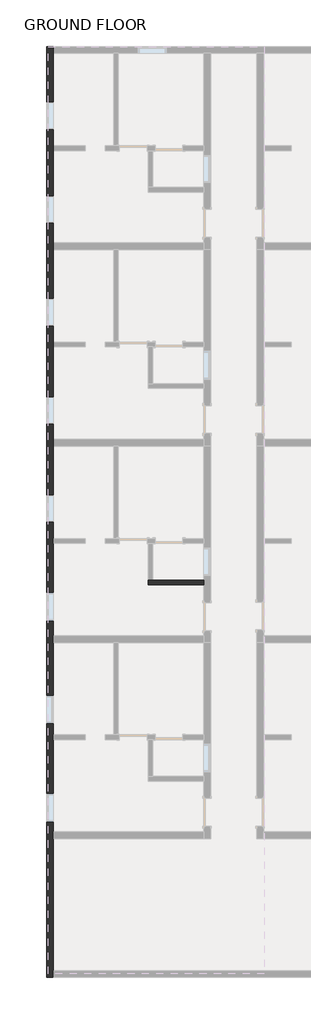
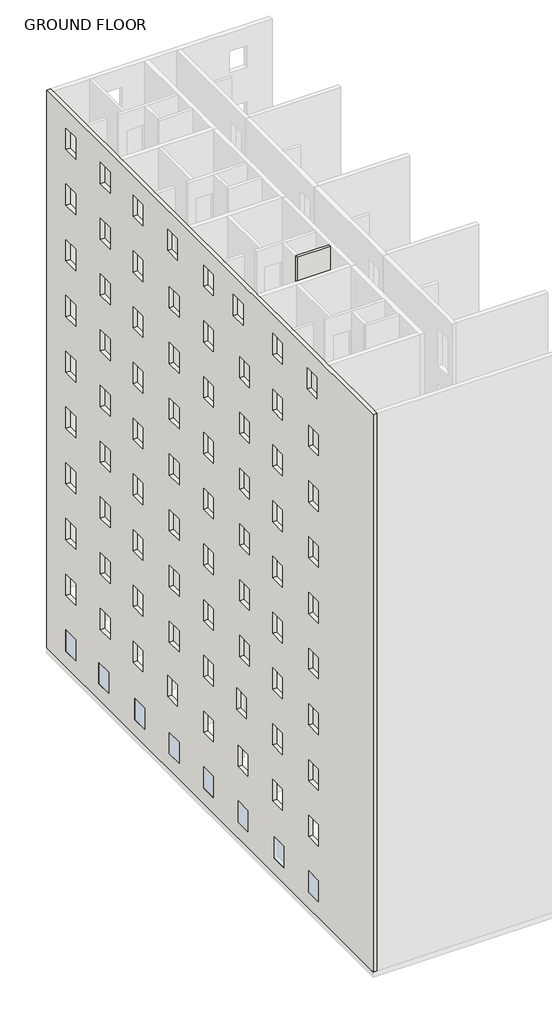
# One storey, part 2 of 7: 2 walls.
"""IFC4 building model written with IfcOpenShell, lengths in millimetres."""

from ifc_helpers import new_model, si_unit, origin, place, context, project, spatial, faceted_brep, element, save

model = new_model("IFC4")

# Units and contexts
model_context = context("Model", 3, world=origin())
ifc_project = project(units=[si_unit("LENGTHUNIT", "METRE", prefix="MILLI")], contexts=[model_context])

# Site, building, storey
site = spatial("IfcSite", under=ifc_project)
building = spatial("IfcBuilding", under=site)
storey = spatial("IfcBuildingStorey", under=building, Name="GROUND FLOOR", Elevation=0.0)

# Walls
placement = place(None, origin())
element("IfcWall", 1, ObjectType="INNER WALL 2", at=placement, inside=storey, context=model_context, shape_type="Brep", body=[
    faceted_brep([(-7539.4902461, -2297.1289408, 0.0), (-9215.8902461, -2297.1289408, 0.0), (-9368.2902461, -2297.1289408, 0.0), (-9368.2902461, -2297.1289408, 32004.0), (-9215.8902461, -2297.1289408, 32004.0), (-7539.4902461, -2297.1289408, 32004.0), (-7539.4902461, -2449.5289408, 0.0), (-7539.4902461, -2449.5289408, 32004.0), (-9368.2902461, -2449.5289408, 32004.0), (-9368.2902461, -2449.5289408, 0.0)], [[[0, 1, 2, 3, 4, 5]], [[6, 7, 8, 9]], [[2, 1, 0, 6, 9]], [[5, 4, 3, 8, 7]], [[0, 5, 7, 6]], [[3, 2, 9, 8]]]),
])
element("IfcWall", 2, ObjectType="OUTER WALL", at=placement, inside=storey, context=model_context, shape_type="Brep", body=[
    faceted_brep([(-12492.4902461, -15403.5289408, 0.0), (-12492.4902461, -15174.9289408, 0.0), (-12492.4902461, -10831.5289408, 0.0), (-12492.4902461, -10602.9289408, 0.0), (-12492.4902461, -7554.9289408, 0.0), (-12492.4902461, -7402.5289408, 0.0), (-12492.4902461, -4354.5289408, 0.0), (-12492.4902461, -4125.9289408, 0.0), (-12492.4902461, -1077.9289408, 0.0), (-12492.4902461, -925.5289408, 0.0), (-12492.4902461, 2122.4710592, 0.0), (-12492.4902461, 2351.0710592, 0.0), (-12492.4902461, 5399.0710592, 0.0), (-12492.4902461, 5551.4710592, 0.0), (-12492.4902461, 8599.4710592, 0.0), (-12492.4902461, 8828.0710592, 0.0), (-12492.4902461, 11876.0710592, 0.0), (-12492.4902461, 12028.4710592, 0.0), (-12492.4902461, 15076.4710592, 0.0), (-12492.4902461, 15305.0710592, 0.0), (-12492.4902461, 15305.0710592, 32004.0), (-12492.4902461, 15076.4710592, 32004.0), (-12492.4902461, 12028.4710592, 32004.0), (-12492.4902461, 11876.0710592, 32004.0), (-12492.4902461, 8828.0710592, 32004.0), (-12492.4902461, 8599.4710592, 32004.0), (-12492.4902461, 5551.4710592, 32004.0), (-12492.4902461, 5399.0710592, 32004.0), (-12492.4902461, 2351.0710592, 32004.0), (-12492.4902461, 2122.4710592, 32004.0), (-12492.4902461, -925.5289408, 32004.0), (-12492.4902461, -1077.9289408, 32004.0), (-12492.4902461, -4125.9289408, 32004.0), (-12492.4902461, -4354.5289408, 32004.0), (-12492.4902461, -7402.5289408, 32004.0), (-12492.4902461, -7554.9289408, 32004.0), (-12492.4902461, -10602.9289408, 32004.0), (-12492.4902461, -10831.5289408, 32004.0), (-12492.4902461, -15174.9289408, 32004.0), (-12492.4902461, -15403.5289408, 32004.0), (-12492.4902461, 13476.2710592, 2133.6), (-12492.4902461, 13476.2710592, 914.4), (-12492.4902461, 12561.8710592, 914.4), (-12492.4902461, 12561.8710592, 2133.6), (-12492.4902461, 10390.1710592, 2133.6), (-12492.4902461, 10390.1710592, 914.4), (-12492.4902461, 9475.7710592, 914.4), (-12492.4902461, 9475.7710592, 2133.6), (-12492.4902461, 6999.2710592, 2133.6), (-12492.4902461, 6999.2710592, 914.4), (-12492.4902461, 6084.8710592, 914.4), (-12492.4902461, 6084.8710592, 2133.6), (-12492.4902461, 3760.7710592, 2133.6), (-12492.4902461, 3760.7710592, 914.4), (-12492.4902461, 2846.3710592, 914.4), (-12492.4902461, 2846.3710592, 2133.6), (-12492.4902461, 522.2710592, 2133.6), (-12492.4902461, 522.2710592, 914.4), (-12492.4902461, -392.1289408, 914.4), (-12492.4902461, -392.1289408, 2133.6), (-12492.4902461, -2716.2289408, 2133.6), (-12492.4902461, -2716.2289408, 914.4), (-12492.4902461, -3630.6289408, 914.4), (-12492.4902461, -3630.6289408, 2133.6), (-12492.4902461, -7021.5289408, 2133.6), (-12492.4902461, -6107.1289408, 2133.6), (-12492.4902461, -6107.1289408, 914.4), (-12492.4902461, -7021.5289408, 914.4), (-12492.4902461, -9345.6289408, 2133.6), (-12492.4902461, -9345.6289408, 914.4), (-12492.4902461, -10260.0289408, 914.4), (-12492.4902461, -10260.0289408, 2133.6), (-12492.4902461, 13476.2710592, 5334.0), (-12492.4902461, 13476.2710592, 4114.8), (-12492.4902461, 12561.8710592, 4114.8), (-12492.4902461, 12561.8710592, 5334.0), (-12492.4902461, 10237.7710592, 5334.0), (-12492.4902461, 10237.7710592, 4114.8), (-12492.4902461, 9323.3710592, 4114.8), (-12492.4902461, 9323.3710592, 5334.0), (-12492.4902461, 7151.6710592, 5334.0), (-12492.4902461, 7151.6710592, 4114.8), (-12492.4902461, 6237.2710592, 4114.8), (-12492.4902461, 6237.2710592, 5334.0), (-12492.4902461, 3913.1710592, 5334.0), (-12492.4902461, 3913.1710592, 4114.8), (-12492.4902461, 2998.7710592, 4114.8), (-12492.4902461, 2998.7710592, 5334.0), (-12492.4902461, 522.2710592, 5334.0), (-12492.4902461, 522.2710592, 4114.8), (-12492.4902461, -392.1289408, 4114.8), (-12492.4902461, -392.1289408, 5334.0), (-12492.4902461, -2716.2289408, 5334.0), (-12492.4902461, -2716.2289408, 4114.8), (-12492.4902461, -3630.6289408, 4114.8), (-12492.4902461, -3630.6289408, 5334.0), (-12492.4902461, -5954.7289408, 5334.0), (-12492.4902461, -5954.7289408, 4114.8), (-12492.4902461, -6869.1289408, 4114.8), (-12492.4902461, -6869.1289408, 5334.0), (-12492.4902461, -9345.6289408, 5334.0), (-12492.4902461, -9345.6289408, 4114.8), (-12492.4902461, -10260.0289408, 4114.8), (-12492.4902461, -10260.0289408, 5334.0), (-12492.4902461, 13476.2710592, 8534.4), (-12492.4902461, 13476.2710592, 7315.2), (-12492.4902461, 12561.8710592, 7315.2), (-12492.4902461, 12561.8710592, 8534.4), (-12492.4902461, 10237.7710592, 8534.4), (-12492.4902461, 10237.7710592, 7315.2), (-12492.4902461, 9323.3710592, 7315.2), (-12492.4902461, 9323.3710592, 8534.4), (-12492.4902461, 7151.6710592, 8534.4), (-12492.4902461, 7151.6710592, 7315.2), (-12492.4902461, 6237.2710592, 7315.2), (-12492.4902461, 6237.2710592, 8534.4), (-12492.4902461, 3760.7710592, 8534.4), (-12492.4902461, 3760.7710592, 7315.2), (-12492.4902461, 2846.3710592, 7315.2), (-12492.4902461, 2846.3710592, 8534.4), (-12492.4902461, 522.2710592, 8534.4), (-12492.4902461, 522.2710592, 7315.2), (-12492.4902461, -392.1289408, 7315.2), (-12492.4902461, -392.1289408, 8534.4), (-12492.4902461, -2563.8289408, 8534.4), (-12492.4902461, -2563.8289408, 7315.2), (-12492.4902461, -3478.2289408, 7315.2), (-12492.4902461, -3478.2289408, 8534.4), (-12492.4902461, -5954.7289408, 8534.4), (-12492.4902461, -5954.7289408, 7315.2), (-12492.4902461, -6869.1289408, 7315.2), (-12492.4902461, -6869.1289408, 8534.4), (-12492.4902461, -9345.6289408, 8534.4), (-12492.4902461, -9345.6289408, 7315.2), (-12492.4902461, -10260.0289408, 7315.2), (-12492.4902461, -10260.0289408, 8534.4), (-12492.4902461, 13476.2710592, 11734.8), (-12492.4902461, 13476.2710592, 10515.6), (-12492.4902461, 12561.8710592, 10515.6), (-12492.4902461, 12561.8710592, 11734.8), (-12492.4902461, 10237.7710592, 11734.8), (-12492.4902461, 10237.7710592, 10515.6), (-12492.4902461, 9323.3710592, 10515.6), (-12492.4902461, 9323.3710592, 11734.8), (-12492.4902461, 7151.6710592, 11734.8), (-12492.4902461, 7151.6710592, 10515.6), (-12492.4902461, 6237.2710592, 10515.6), (-12492.4902461, 6237.2710592, 11734.8), (-12492.4902461, 3760.7710592, 11734.8), (-12492.4902461, 3760.7710592, 10515.6), (-12492.4902461, 2846.3710592, 10515.6), (-12492.4902461, 2846.3710592, 11734.8), (-12492.4902461, 522.2710592, 11734.8), (-12492.4902461, 522.2710592, 10515.6), (-12492.4902461, -392.1289408, 10515.6), (-12492.4902461, -392.1289408, 11734.8), (-12492.4902461, -2868.6289408, 11734.8), (-12492.4902461, -2868.6289408, 10515.6), (-12492.4902461, -3783.0289408, 10515.6), (-12492.4902461, -3783.0289408, 11734.8), (-12492.4902461, -5954.7289408, 11734.8), (-12492.4902461, -5954.7289408, 10515.6), (-12492.4902461, -6869.1289408, 10515.6), (-12492.4902461, -6869.1289408, 11734.8), (-12492.4902461, -9345.6289408, 11734.8), (-12492.4902461, -9345.6289408, 10515.6), (-12492.4902461, -10260.0289408, 10515.6), (-12492.4902461, -10260.0289408, 11734.8), (-12492.4902461, -9345.6289408, 14935.2), (-12492.4902461, -9345.6289408, 13716.0), (-12492.4902461, -10260.0289408, 13716.0), (-12492.4902461, -10260.0289408, 14935.2), (-12492.4902461, -5954.7289408, 14935.2), (-12492.4902461, -5954.7289408, 13716.0), (-12492.4902461, -6869.1289408, 13716.0), (-12492.4902461, -6869.1289408, 14935.2), (-12492.4902461, -2868.6289408, 14935.2), (-12492.4902461, -2868.6289408, 13716.0), (-12492.4902461, -3783.0289408, 13716.0), (-12492.4902461, -3783.0289408, 14935.2), (-12492.4902461, 522.2710592, 14935.2), (-12492.4902461, 522.2710592, 13716.0), (-12492.4902461, -392.1289408, 13716.0), (-12492.4902461, -392.1289408, 14935.2), (-12492.4902461, 3760.7710592, 14935.2), (-12492.4902461, 3760.7710592, 13716.0), (-12492.4902461, 2846.3710592, 13716.0), (-12492.4902461, 2846.3710592, 14935.2), (-12492.4902461, 7151.6710592, 14935.2), (-12492.4902461, 7151.6710592, 13716.0), (-12492.4902461, 6237.2710592, 13716.0), (-12492.4902461, 6237.2710592, 14935.2), (-12492.4902461, 10237.7710592, 14935.2), (-12492.4902461, 10237.7710592, 13716.0), (-12492.4902461, 9323.3710592, 13716.0), (-12492.4902461, 9323.3710592, 14935.2), (-12492.4902461, 13476.2710592, 14935.2), (-12492.4902461, 13476.2710592, 13716.0), (-12492.4902461, 12561.8710592, 13716.0), (-12492.4902461, 12561.8710592, 14935.2), (-12492.4902461, 13476.2710592, 18135.6), (-12492.4902461, 13476.2710592, 16916.4), (-12492.4902461, 12561.8710592, 16916.4), (-12492.4902461, 12561.8710592, 18135.6), (-12492.4902461, 10237.7710592, 18135.6), (-12492.4902461, 10237.7710592, 16916.4), (-12492.4902461, 9323.3710592, 16916.4), (-12492.4902461, 9323.3710592, 18135.6), (-12492.4902461, 7151.6710592, 18135.6), (-12492.4902461, 7151.6710592, 16916.4), (-12492.4902461, 6237.2710592, 16916.4), (-12492.4902461, 6237.2710592, 18135.6), (-12492.4902461, 3760.7710592, 18135.6), (-12492.4902461, 3760.7710592, 16916.4), (-12492.4902461, 2846.3710592, 16916.4), (-12492.4902461, 2846.3710592, 18135.6), (-12492.4902461, 522.2710592, 18135.6), (-12492.4902461, 522.2710592, 16916.4), (-12492.4902461, -392.1289408, 16916.4), (-12492.4902461, -392.1289408, 18135.6), (-12492.4902461, -2868.6289408, 18135.6), (-12492.4902461, -2868.6289408, 16916.4), (-12492.4902461, -3783.0289408, 16916.4), (-12492.4902461, -3783.0289408, 18135.6), (-12492.4902461, -5954.7289408, 18135.6), (-12492.4902461, -5954.7289408, 16916.4), (-12492.4902461, -6869.1289408, 16916.4), (-12492.4902461, -6869.1289408, 18135.6), (-12492.4902461, -9345.6289408, 18135.6), (-12492.4902461, -9345.6289408, 16916.4), (-12492.4902461, -10260.0289408, 16916.4), (-12492.4902461, -10260.0289408, 18135.6), (-12492.4902461, -9345.6289408, 21336.0), (-12492.4902461, -9345.6289408, 20116.8), (-12492.4902461, -10260.0289408, 20116.8), (-12492.4902461, -10260.0289408, 21336.0), (-12492.4902461, -5954.7289408, 21336.0), (-12492.4902461, -5954.7289408, 20116.8), (-12492.4902461, -6869.1289408, 20116.8), (-12492.4902461, -6869.1289408, 21336.0), (-12492.4902461, -2868.6289408, 21336.0), (-12492.4902461, -2868.6289408, 20116.8), (-12492.4902461, -3783.0289408, 20116.8), (-12492.4902461, -3783.0289408, 21336.0), (-12492.4902461, 522.2710592, 21336.0), (-12492.4902461, 522.2710592, 20116.8), (-12492.4902461, -392.1289408, 20116.8), (-12492.4902461, -392.1289408, 21336.0), (-12492.4902461, 3760.7710592, 21336.0), (-12492.4902461, 3760.7710592, 20116.8), (-12492.4902461, 2846.3710592, 20116.8), (-12492.4902461, 2846.3710592, 21336.0), (-12492.4902461, 7151.6710592, 21336.0), (-12492.4902461, 7151.6710592, 20116.8), (-12492.4902461, 6237.2710592, 20116.8), (-12492.4902461, 6237.2710592, 21336.0), (-12492.4902461, 10237.7710592, 21336.0), (-12492.4902461, 10237.7710592, 20116.8), (-12492.4902461, 9323.3710592, 20116.8), (-12492.4902461, 9323.3710592, 21336.0), (-12492.4902461, 13476.2710592, 21336.0), (-12492.4902461, 13476.2710592, 20116.8), (-12492.4902461, 12561.8710592, 20116.8), (-12492.4902461, 12561.8710592, 21336.0), (-12492.4902461, -9345.6289408, 24536.4), (-12492.4902461, -9345.6289408, 23317.2), (-12492.4902461, -10260.0289408, 23317.2), (-12492.4902461, -10260.0289408, 24536.4), (-12492.4902461, -5954.7289408, 24536.4), (-12492.4902461, -5954.7289408, 23317.2), (-12492.4902461, -6869.1289408, 23317.2), (-12492.4902461, -6869.1289408, 24536.4), (-12492.4902461, -2868.6289408, 24536.4), (-12492.4902461, -2868.6289408, 23317.2), (-12492.4902461, -3783.0289408, 23317.2), (-12492.4902461, -3783.0289408, 24536.4), (-12492.4902461, 522.2710592, 24536.4), (-12492.4902461, 522.2710592, 23317.2), (-12492.4902461, -392.1289408, 23317.2), (-12492.4902461, -392.1289408, 24536.4), (-12492.4902461, 3760.7710592, 24536.4), (-12492.4902461, 3760.7710592, 23317.2), (-12492.4902461, 2846.3710592, 23317.2), (-12492.4902461, 2846.3710592, 24536.4), (-12492.4902461, 7151.6710592, 24536.4), (-12492.4902461, 7151.6710592, 23317.2), (-12492.4902461, 6237.2710592, 23317.2), (-12492.4902461, 6237.2710592, 24536.4), (-12492.4902461, 10237.7710592, 24536.4), (-12492.4902461, 10237.7710592, 23317.2), (-12492.4902461, 9323.3710592, 23317.2), (-12492.4902461, 9323.3710592, 24536.4), (-12492.4902461, 13476.2710592, 24536.4), (-12492.4902461, 13476.2710592, 23317.2), (-12492.4902461, 12561.8710592, 23317.2), (-12492.4902461, 12561.8710592, 24536.4), (-12492.4902461, 10237.7710592, 27736.8), (-12492.4902461, 10237.7710592, 26517.6), (-12492.4902461, 9323.3710592, 26517.6), (-12492.4902461, 9323.3710592, 27736.8), (-12492.4902461, 13476.2710592, 27736.8), (-12492.4902461, 13476.2710592, 26517.6), (-12492.4902461, 12561.8710592, 26517.6), (-12492.4902461, 12561.8710592, 27736.8), (-12492.4902461, 7151.6710592, 27736.8), (-12492.4902461, 7151.6710592, 26517.6), (-12492.4902461, 6237.2710592, 26517.6), (-12492.4902461, 6237.2710592, 27736.8), (-12492.4902461, 3760.7710592, 27736.8), (-12492.4902461, 3760.7710592, 26517.6), (-12492.4902461, 2846.3710592, 26517.6), (-12492.4902461, 2846.3710592, 27736.8), (-12492.4902461, 522.2710592, 27736.8), (-12492.4902461, 522.2710592, 26517.6), (-12492.4902461, -392.1289408, 26517.6), (-12492.4902461, -392.1289408, 27736.8), (-12492.4902461, -2868.6289408, 27736.8), (-12492.4902461, -2868.6289408, 26517.6), (-12492.4902461, -3783.0289408, 26517.6), (-12492.4902461, -3783.0289408, 27736.8), (-12492.4902461, -5954.7289408, 27736.8), (-12492.4902461, -5954.7289408, 26517.6), (-12492.4902461, -6869.1289408, 26517.6), (-12492.4902461, -6869.1289408, 27736.8), (-12492.4902461, -9345.6289408, 27736.8), (-12492.4902461, -9345.6289408, 26517.6), (-12492.4902461, -10260.0289408, 26517.6), (-12492.4902461, -10260.0289408, 27736.8), (-12492.4902461, -9193.2289408, 30937.2), (-12492.4902461, -9193.2289408, 29718.0), (-12492.4902461, -10107.6289408, 29718.0), (-12492.4902461, -10107.6289408, 30937.2), (-12492.4902461, -5954.7289408, 30937.2), (-12492.4902461, -5954.7289408, 29718.0), (-12492.4902461, -6869.1289408, 29718.0), (-12492.4902461, -6869.1289408, 30937.2), (-12492.4902461, -2259.0289408, 30937.2), (-12492.4902461, -2259.0289408, 29718.0), (-12492.4902461, -3173.4289408, 29718.0), (-12492.4902461, -3173.4289408, 30937.2), (-12492.4902461, 522.2710592, 30937.2), (-12492.4902461, 522.2710592, 29718.0), (-12492.4902461, -392.1289408, 29718.0), (-12492.4902461, -392.1289408, 30937.2), (-12492.4902461, 3913.1710592, 30937.2), (-12492.4902461, 3913.1710592, 29718.0), (-12492.4902461, 2998.7710592, 29718.0), (-12492.4902461, 2998.7710592, 30937.2), (-12492.4902461, 7151.6710592, 30937.2), (-12492.4902461, 7151.6710592, 29718.0), (-12492.4902461, 6237.2710592, 29718.0), (-12492.4902461, 6237.2710592, 30937.2), (-12492.4902461, 10237.7710592, 30937.2), (-12492.4902461, 10237.7710592, 29718.0), (-12492.4902461, 9323.3710592, 29718.0), (-12492.4902461, 9323.3710592, 30937.2), (-12492.4902461, 13476.2710592, 30937.2), (-12492.4902461, 13476.2710592, 29718.0), (-12492.4902461, 12561.8710592, 29718.0), (-12492.4902461, 12561.8710592, 30937.2), (-12721.0902461, -15403.5289408, 0.0), (-12721.0902461, -15403.5289408, 32004.0), (-12721.0902461, 15305.0710592, 32004.0), (-12721.0902461, 15305.0710592, 0.0), (-12721.0902461, 13476.2710592, 2133.6), (-12721.0902461, 12561.8710592, 2133.6), (-12721.0902461, 12561.8710592, 914.4), (-12721.0902461, 13476.2710592, 914.4), (-12721.0902461, 10390.1710592, 2133.6), (-12721.0902461, 9475.7710592, 2133.6), (-12721.0902461, 9475.7710592, 914.4), (-12721.0902461, 10390.1710592, 914.4), (-12721.0902461, 6999.2710592, 2133.6), (-12721.0902461, 6084.8710592, 2133.6), (-12721.0902461, 6084.8710592, 914.4), (-12721.0902461, 6999.2710592, 914.4), (-12721.0902461, 3760.7710592, 2133.6), (-12721.0902461, 2846.3710592, 2133.6), (-12721.0902461, 2846.3710592, 914.4), (-12721.0902461, 3760.7710592, 914.4), (-12721.0902461, 522.2710592, 2133.6), (-12721.0902461, -392.1289408, 2133.6), (-12721.0902461, -392.1289408, 914.4), (-12721.0902461, 522.2710592, 914.4), (-12721.0902461, -2716.2289408, 2133.6), (-12721.0902461, -3630.6289408, 2133.6), (-12721.0902461, -3630.6289408, 914.4), (-12721.0902461, -2716.2289408, 914.4), (-12721.0902461, -7021.5289408, 2133.6), (-12721.0902461, -7021.5289408, 914.4), (-12721.0902461, -6107.1289408, 914.4), (-12721.0902461, -6107.1289408, 2133.6), (-12721.0902461, -9345.6289408, 2133.6), (-12721.0902461, -10260.0289408, 2133.6), (-12721.0902461, -10260.0289408, 914.4), (-12721.0902461, -9345.6289408, 914.4), (-12721.0902461, 13476.2710592, 5334.0), (-12721.0902461, 12561.8710592, 5334.0), (-12721.0902461, 12561.8710592, 4114.8), (-12721.0902461, 13476.2710592, 4114.8), (-12721.0902461, 10237.7710592, 5334.0), (-12721.0902461, 9323.3710592, 5334.0), (-12721.0902461, 9323.3710592, 4114.8), (-12721.0902461, 10237.7710592, 4114.8), (-12721.0902461, 7151.6710592, 5334.0), (-12721.0902461, 6237.2710592, 5334.0), (-12721.0902461, 6237.2710592, 4114.8), (-12721.0902461, 7151.6710592, 4114.8), (-12721.0902461, 3913.1710592, 5334.0), (-12721.0902461, 2998.7710592, 5334.0), (-12721.0902461, 2998.7710592, 4114.8), (-12721.0902461, 3913.1710592, 4114.8), (-12721.0902461, 522.2710592, 5334.0), (-12721.0902461, -392.1289408, 5334.0), (-12721.0902461, -392.1289408, 4114.8), (-12721.0902461, 522.2710592, 4114.8), (-12721.0902461, -2716.2289408, 5334.0), (-12721.0902461, -3630.6289408, 5334.0), (-12721.0902461, -3630.6289408, 4114.8), (-12721.0902461, -2716.2289408, 4114.8), (-12721.0902461, -5954.7289408, 5334.0), (-12721.0902461, -6869.1289408, 5334.0), (-12721.0902461, -6869.1289408, 4114.8), (-12721.0902461, -5954.7289408, 4114.8), (-12721.0902461, -9345.6289408, 5334.0), (-12721.0902461, -10260.0289408, 5334.0), (-12721.0902461, -10260.0289408, 4114.8), (-12721.0902461, -9345.6289408, 4114.8), (-12721.0902461, 13476.2710592, 8534.4), (-12721.0902461, 12561.8710592, 8534.4), (-12721.0902461, 12561.8710592, 7315.2), (-12721.0902461, 13476.2710592, 7315.2), (-12721.0902461, 10237.7710592, 8534.4), (-12721.0902461, 9323.3710592, 8534.4), (-12721.0902461, 9323.3710592, 7315.2), (-12721.0902461, 10237.7710592, 7315.2), (-12721.0902461, 7151.6710592, 8534.4), (-12721.0902461, 6237.2710592, 8534.4), (-12721.0902461, 6237.2710592, 7315.2), (-12721.0902461, 7151.6710592, 7315.2), (-12721.0902461, 3760.7710592, 8534.4), (-12721.0902461, 2846.3710592, 8534.4), (-12721.0902461, 2846.3710592, 7315.2), (-12721.0902461, 3760.7710592, 7315.2), (-12721.0902461, 522.2710592, 8534.4), (-12721.0902461, -392.1289408, 8534.4), (-12721.0902461, -392.1289408, 7315.2), (-12721.0902461, 522.2710592, 7315.2), (-12721.0902461, -2563.8289408, 8534.4), (-12721.0902461, -3478.2289408, 8534.4), (-12721.0902461, -3478.2289408, 7315.2), (-12721.0902461, -2563.8289408, 7315.2), (-12721.0902461, -5954.7289408, 8534.4), (-12721.0902461, -6869.1289408, 8534.4), (-12721.0902461, -6869.1289408, 7315.2), (-12721.0902461, -5954.7289408, 7315.2), (-12721.0902461, -9345.6289408, 8534.4), (-12721.0902461, -10260.0289408, 8534.4), (-12721.0902461, -10260.0289408, 7315.2), (-12721.0902461, -9345.6289408, 7315.2), (-12721.0902461, 13476.2710592, 11734.8), (-12721.0902461, 12561.8710592, 11734.8), (-12721.0902461, 12561.8710592, 10515.6), (-12721.0902461, 13476.2710592, 10515.6), (-12721.0902461, 10237.7710592, 11734.8), (-12721.0902461, 9323.3710592, 11734.8), (-12721.0902461, 9323.3710592, 10515.6), (-12721.0902461, 10237.7710592, 10515.6), (-12721.0902461, 7151.6710592, 11734.8), (-12721.0902461, 6237.2710592, 11734.8), (-12721.0902461, 6237.2710592, 10515.6), (-12721.0902461, 7151.6710592, 10515.6), (-12721.0902461, 3760.7710592, 11734.8), (-12721.0902461, 2846.3710592, 11734.8), (-12721.0902461, 2846.3710592, 10515.6), (-12721.0902461, 3760.7710592, 10515.6), (-12721.0902461, 522.2710592, 11734.8), (-12721.0902461, -392.1289408, 11734.8), (-12721.0902461, -392.1289408, 10515.6), (-12721.0902461, 522.2710592, 10515.6), (-12721.0902461, -2868.6289408, 11734.8), (-12721.0902461, -3783.0289408, 11734.8), (-12721.0902461, -3783.0289408, 10515.6), (-12721.0902461, -2868.6289408, 10515.6), (-12721.0902461, -5954.7289408, 11734.8), (-12721.0902461, -6869.1289408, 11734.8), (-12721.0902461, -6869.1289408, 10515.6), (-12721.0902461, -5954.7289408, 10515.6), (-12721.0902461, -9345.6289408, 11734.8), (-12721.0902461, -10260.0289408, 11734.8), (-12721.0902461, -10260.0289408, 10515.6), (-12721.0902461, -9345.6289408, 10515.6), (-12721.0902461, -9345.6289408, 14935.2), (-12721.0902461, -10260.0289408, 14935.2), (-12721.0902461, -10260.0289408, 13716.0), (-12721.0902461, -9345.6289408, 13716.0), (-12721.0902461, -5954.7289408, 14935.2), (-12721.0902461, -6869.1289408, 14935.2), (-12721.0902461, -6869.1289408, 13716.0), (-12721.0902461, -5954.7289408, 13716.0), (-12721.0902461, -2868.6289408, 14935.2), (-12721.0902461, -3783.0289408, 14935.2), (-12721.0902461, -3783.0289408, 13716.0), (-12721.0902461, -2868.6289408, 13716.0), (-12721.0902461, 522.2710592, 14935.2), (-12721.0902461, -392.1289408, 14935.2), (-12721.0902461, -392.1289408, 13716.0), (-12721.0902461, 522.2710592, 13716.0), (-12721.0902461, 3760.7710592, 14935.2), (-12721.0902461, 2846.3710592, 14935.2), (-12721.0902461, 2846.3710592, 13716.0), (-12721.0902461, 3760.7710592, 13716.0), (-12721.0902461, 7151.6710592, 14935.2), (-12721.0902461, 6237.2710592, 14935.2), (-12721.0902461, 6237.2710592, 13716.0), (-12721.0902461, 7151.6710592, 13716.0), (-12721.0902461, 10237.7710592, 14935.2), (-12721.0902461, 9323.3710592, 14935.2), (-12721.0902461, 9323.3710592, 13716.0), (-12721.0902461, 10237.7710592, 13716.0), (-12721.0902461, 13476.2710592, 14935.2), (-12721.0902461, 12561.8710592, 14935.2), (-12721.0902461, 12561.8710592, 13716.0), (-12721.0902461, 13476.2710592, 13716.0), (-12721.0902461, 13476.2710592, 18135.6), (-12721.0902461, 12561.8710592, 18135.6), (-12721.0902461, 12561.8710592, 16916.4), (-12721.0902461, 13476.2710592, 16916.4), (-12721.0902461, 10237.7710592, 18135.6), (-12721.0902461, 9323.3710592, 18135.6), (-12721.0902461, 9323.3710592, 16916.4), (-12721.0902461, 10237.7710592, 16916.4), (-12721.0902461, 7151.6710592, 18135.6), (-12721.0902461, 6237.2710592, 18135.6), (-12721.0902461, 6237.2710592, 16916.4), (-12721.0902461, 7151.6710592, 16916.4), (-12721.0902461, 3760.7710592, 18135.6), (-12721.0902461, 2846.3710592, 18135.6), (-12721.0902461, 2846.3710592, 16916.4), (-12721.0902461, 3760.7710592, 16916.4), (-12721.0902461, 522.2710592, 18135.6), (-12721.0902461, -392.1289408, 18135.6), (-12721.0902461, -392.1289408, 16916.4), (-12721.0902461, 522.2710592, 16916.4), (-12721.0902461, -2868.6289408, 18135.6), (-12721.0902461, -3783.0289408, 18135.6), (-12721.0902461, -3783.0289408, 16916.4), (-12721.0902461, -2868.6289408, 16916.4), (-12721.0902461, -5954.7289408, 18135.6), (-12721.0902461, -6869.1289408, 18135.6), (-12721.0902461, -6869.1289408, 16916.4), (-12721.0902461, -5954.7289408, 16916.4), (-12721.0902461, -9345.6289408, 18135.6), (-12721.0902461, -10260.0289408, 18135.6), (-12721.0902461, -10260.0289408, 16916.4), (-12721.0902461, -9345.6289408, 16916.4), (-12721.0902461, -9345.6289408, 21336.0), (-12721.0902461, -10260.0289408, 21336.0), (-12721.0902461, -10260.0289408, 20116.8), (-12721.0902461, -9345.6289408, 20116.8), (-12721.0902461, -5954.7289408, 21336.0), (-12721.0902461, -6869.1289408, 21336.0), (-12721.0902461, -6869.1289408, 20116.8), (-12721.0902461, -5954.7289408, 20116.8), (-12721.0902461, -2868.6289408, 21336.0), (-12721.0902461, -3783.0289408, 21336.0), (-12721.0902461, -3783.0289408, 20116.8), (-12721.0902461, -2868.6289408, 20116.8), (-12721.0902461, 522.2710592, 21336.0), (-12721.0902461, -392.1289408, 21336.0), (-12721.0902461, -392.1289408, 20116.8), (-12721.0902461, 522.2710592, 20116.8), (-12721.0902461, 3760.7710592, 21336.0), (-12721.0902461, 2846.3710592, 21336.0), (-12721.0902461, 2846.3710592, 20116.8), (-12721.0902461, 3760.7710592, 20116.8), (-12721.0902461, 7151.6710592, 21336.0), (-12721.0902461, 6237.2710592, 21336.0), (-12721.0902461, 6237.2710592, 20116.8), (-12721.0902461, 7151.6710592, 20116.8), (-12721.0902461, 10237.7710592, 21336.0), (-12721.0902461, 9323.3710592, 21336.0), (-12721.0902461, 9323.3710592, 20116.8), (-12721.0902461, 10237.7710592, 20116.8), (-12721.0902461, 13476.2710592, 21336.0), (-12721.0902461, 12561.8710592, 21336.0), (-12721.0902461, 12561.8710592, 20116.8), (-12721.0902461, 13476.2710592, 20116.8), (-12721.0902461, -9345.6289408, 24536.4), (-12721.0902461, -10260.0289408, 24536.4), (-12721.0902461, -10260.0289408, 23317.2), (-12721.0902461, -9345.6289408, 23317.2), (-12721.0902461, -5954.7289408, 24536.4), (-12721.0902461, -6869.1289408, 24536.4), (-12721.0902461, -6869.1289408, 23317.2), (-12721.0902461, -5954.7289408, 23317.2), (-12721.0902461, -2868.6289408, 24536.4), (-12721.0902461, -3783.0289408, 24536.4), (-12721.0902461, -3783.0289408, 23317.2), (-12721.0902461, -2868.6289408, 23317.2), (-12721.0902461, 522.2710592, 24536.4), (-12721.0902461, -392.1289408, 24536.4), (-12721.0902461, -392.1289408, 23317.2), (-12721.0902461, 522.2710592, 23317.2), (-12721.0902461, 3760.7710592, 24536.4), (-12721.0902461, 2846.3710592, 24536.4), (-12721.0902461, 2846.3710592, 23317.2), (-12721.0902461, 3760.7710592, 23317.2), (-12721.0902461, 7151.6710592, 24536.4), (-12721.0902461, 6237.2710592, 24536.4), (-12721.0902461, 6237.2710592, 23317.2), (-12721.0902461, 7151.6710592, 23317.2), (-12721.0902461, 10237.7710592, 24536.4), (-12721.0902461, 9323.3710592, 24536.4), (-12721.0902461, 9323.3710592, 23317.2), (-12721.0902461, 10237.7710592, 23317.2), (-12721.0902461, 13476.2710592, 24536.4), (-12721.0902461, 12561.8710592, 24536.4), (-12721.0902461, 12561.8710592, 23317.2), (-12721.0902461, 13476.2710592, 23317.2), (-12721.0902461, 10237.7710592, 27736.8), (-12721.0902461, 9323.3710592, 27736.8), (-12721.0902461, 9323.3710592, 26517.6), (-12721.0902461, 10237.7710592, 26517.6), (-12721.0902461, 13476.2710592, 27736.8), (-12721.0902461, 12561.8710592, 27736.8), (-12721.0902461, 12561.8710592, 26517.6), (-12721.0902461, 13476.2710592, 26517.6), (-12721.0902461, 7151.6710592, 27736.8), (-12721.0902461, 6237.2710592, 27736.8), (-12721.0902461, 6237.2710592, 26517.6), (-12721.0902461, 7151.6710592, 26517.6), (-12721.0902461, 3760.7710592, 27736.8), (-12721.0902461, 2846.3710592, 27736.8), (-12721.0902461, 2846.3710592, 26517.6), (-12721.0902461, 3760.7710592, 26517.6), (-12721.0902461, 522.2710592, 27736.8), (-12721.0902461, -392.1289408, 27736.8), (-12721.0902461, -392.1289408, 26517.6), (-12721.0902461, 522.2710592, 26517.6), (-12721.0902461, -2868.6289408, 27736.8), (-12721.0902461, -3783.0289408, 27736.8), (-12721.0902461, -3783.0289408, 26517.6), (-12721.0902461, -2868.6289408, 26517.6), (-12721.0902461, -5954.7289408, 27736.8), (-12721.0902461, -6869.1289408, 27736.8), (-12721.0902461, -6869.1289408, 26517.6), (-12721.0902461, -5954.7289408, 26517.6), (-12721.0902461, -9345.6289408, 27736.8), (-12721.0902461, -10260.0289408, 27736.8), (-12721.0902461, -10260.0289408, 26517.6), (-12721.0902461, -9345.6289408, 26517.6), (-12721.0902461, -9193.2289408, 30937.2), (-12721.0902461, -10107.6289408, 30937.2), (-12721.0902461, -10107.6289408, 29718.0), (-12721.0902461, -9193.2289408, 29718.0), (-12721.0902461, -5954.7289408, 30937.2), (-12721.0902461, -6869.1289408, 30937.2), (-12721.0902461, -6869.1289408, 29718.0), (-12721.0902461, -5954.7289408, 29718.0), (-12721.0902461, -2259.0289408, 30937.2), (-12721.0902461, -3173.4289408, 30937.2), (-12721.0902461, -3173.4289408, 29718.0), (-12721.0902461, -2259.0289408, 29718.0), (-12721.0902461, 522.2710592, 30937.2), (-12721.0902461, -392.1289408, 30937.2), (-12721.0902461, -392.1289408, 29718.0), (-12721.0902461, 522.2710592, 29718.0), (-12721.0902461, 3913.1710592, 30937.2), (-12721.0902461, 2998.7710592, 30937.2), (-12721.0902461, 2998.7710592, 29718.0), (-12721.0902461, 3913.1710592, 29718.0), (-12721.0902461, 7151.6710592, 30937.2), (-12721.0902461, 6237.2710592, 30937.2), (-12721.0902461, 6237.2710592, 29718.0), (-12721.0902461, 7151.6710592, 29718.0), (-12721.0902461, 10237.7710592, 30937.2), (-12721.0902461, 9323.3710592, 30937.2), (-12721.0902461, 9323.3710592, 29718.0), (-12721.0902461, 10237.7710592, 29718.0), (-12721.0902461, 13476.2710592, 30937.2), (-12721.0902461, 12561.8710592, 30937.2), (-12721.0902461, 12561.8710592, 29718.0), (-12721.0902461, 13476.2710592, 29718.0)], [[[0, 1, 2, 3, 4, 5, 6, 7, 8, 9, 10, 11, 12, 13, 14, 15, 16, 17, 18, 19, 20, 21, 22, 23, 24, 25, 26, 27, 28, 29, 30, 31, 32, 33, 34, 35, 36, 37, 38, 39], [40, 41, 42, 43], [44, 45, 46, 47], [48, 49, 50, 51], [52, 53, 54, 55], [56, 57, 58, 59], [60, 61, 62, 63], [64, 65, 66, 67], [68, 69, 70, 71], [72, 73, 74, 75], [76, 77, 78, 79], [80, 81, 82, 83], [84, 85, 86, 87], [88, 89, 90, 91], [92, 93, 94, 95], [96, 97, 98, 99], [100, 101, 102, 103], [104, 105, 106, 107], [108, 109, 110, 111], [112, 113, 114, 115], [116, 117, 118, 119], [120, 121, 122, 123], [124, 125, 126, 127], [128, 129, 130, 131], [132, 133, 134, 135], [136, 137, 138, 139], [140, 141, 142, 143], [144, 145, 146, 147], [148, 149, 150, 151], [152, 153, 154, 155], [156, 157, 158, 159], [160, 161, 162, 163], [164, 165, 166, 167], [168, 169, 170, 171], [172, 173, 174, 175], [176, 177, 178, 179], [180, 181, 182, 183], [184, 185, 186, 187], [188, 189, 190, 191], [192, 193, 194, 195], [196, 197, 198, 199], [200, 201, 202, 203], [204, 205, 206, 207], [208, 209, 210, 211], [212, 213, 214, 215], [216, 217, 218, 219], [220, 221, 222, 223], [224, 225, 226, 227], [228, 229, 230, 231], [232, 233, 234, 235], [236, 237, 238, 239], [240, 241, 242, 243], [244, 245, 246, 247], [248, 249, 250, 251], [252, 253, 254, 255], [256, 257, 258, 259], [260, 261, 262, 263], [264, 265, 266, 267], [268, 269, 270, 271], [272, 273, 274, 275], [276, 277, 278, 279], [280, 281, 282, 283], [284, 285, 286, 287], [288, 289, 290, 291], [292, 293, 294, 295], [296, 297, 298, 299], [300, 301, 302, 303], [304, 305, 306, 307], [308, 309, 310, 311], [312, 313, 314, 315], [316, 317, 318, 319], [320, 321, 322, 323], [324, 325, 326, 327], [328, 329, 330, 331], [332, 333, 334, 335], [336, 337, 338, 339], [340, 341, 342, 343], [344, 345, 346, 347], [348, 349, 350, 351], [352, 353, 354, 355], [356, 357, 358, 359]], [[360, 361, 362, 363], [364, 365, 366, 367], [368, 369, 370, 371], [372, 373, 374, 375], [376, 377, 378, 379], [380, 381, 382, 383], [384, 385, 386, 387], [388, 389, 390, 391], [392, 393, 394, 395], [396, 397, 398, 399], [400, 401, 402, 403], [404, 405, 406, 407], [408, 409, 410, 411], [412, 413, 414, 415], [416, 417, 418, 419], [420, 421, 422, 423], [424, 425, 426, 427], [428, 429, 430, 431], [432, 433, 434, 435], [436, 437, 438, 439], [440, 441, 442, 443], [444, 445, 446, 447], [448, 449, 450, 451], [452, 453, 454, 455], [456, 457, 458, 459], [460, 461, 462, 463], [464, 465, 466, 467], [468, 469, 470, 471], [472, 473, 474, 475], [476, 477, 478, 479], [480, 481, 482, 483], [484, 485, 486, 487], [488, 489, 490, 491], [492, 493, 494, 495], [496, 497, 498, 499], [500, 501, 502, 503], [504, 505, 506, 507], [508, 509, 510, 511], [512, 513, 514, 515], [516, 517, 518, 519], [520, 521, 522, 523], [524, 525, 526, 527], [528, 529, 530, 531], [532, 533, 534, 535], [536, 537, 538, 539], [540, 541, 542, 543], [544, 545, 546, 547], [548, 549, 550, 551], [552, 553, 554, 555], [556, 557, 558, 559], [560, 561, 562, 563], [564, 565, 566, 567], [568, 569, 570, 571], [572, 573, 574, 575], [576, 577, 578, 579], [580, 581, 582, 583], [584, 585, 586, 587], [588, 589, 590, 591], [592, 593, 594, 595], [596, 597, 598, 599], [600, 601, 602, 603], [604, 605, 606, 607], [608, 609, 610, 611], [612, 613, 614, 615], [616, 617, 618, 619], [620, 621, 622, 623], [624, 625, 626, 627], [628, 629, 630, 631], [632, 633, 634, 635], [636, 637, 638, 639], [640, 641, 642, 643], [644, 645, 646, 647], [648, 649, 650, 651], [652, 653, 654, 655], [656, 657, 658, 659], [660, 661, 662, 663], [664, 665, 666, 667], [668, 669, 670, 671], [672, 673, 674, 675], [676, 677, 678, 679], [680, 681, 682, 683]], [[19, 18, 17, 16, 15, 14, 13, 12, 11, 10, 9, 8, 7, 6, 5, 4, 3, 2, 1, 0, 360, 363]], [[39, 38, 37, 36, 35, 34, 33, 32, 31, 30, 29, 28, 27, 26, 25, 24, 23, 22, 21, 20, 362, 361]], [[41, 40, 364, 367]], [[42, 41, 367, 366]], [[43, 42, 366, 365]], [[40, 43, 365, 364]], [[45, 44, 368, 371]], [[46, 45, 371, 370]], [[47, 46, 370, 369]], [[44, 47, 369, 368]], [[49, 48, 372, 375]], [[50, 49, 375, 374]], [[51, 50, 374, 373]], [[48, 51, 373, 372]], [[53, 52, 376, 379]], [[54, 53, 379, 378]], [[55, 54, 378, 377]], [[52, 55, 377, 376]], [[57, 56, 380, 383]], [[58, 57, 383, 382]], [[59, 58, 382, 381]], [[56, 59, 381, 380]], [[61, 60, 384, 387]], [[62, 61, 387, 386]], [[63, 62, 386, 385]], [[60, 63, 385, 384]], [[389, 388, 64, 67]], [[390, 389, 67, 66]], [[391, 390, 66, 65]], [[388, 391, 65, 64]], [[69, 68, 392, 395]], [[70, 69, 395, 394]], [[71, 70, 394, 393]], [[68, 71, 393, 392]], [[20, 19, 363, 362]], [[73, 72, 396, 399]], [[74, 73, 399, 398]], [[75, 74, 398, 397]], [[72, 75, 397, 396]], [[77, 76, 400, 403]], [[78, 77, 403, 402]], [[79, 78, 402, 401]], [[76, 79, 401, 400]], [[81, 80, 404, 407]], [[82, 81, 407, 406]], [[83, 82, 406, 405]], [[80, 83, 405, 404]], [[85, 84, 408, 411]], [[86, 85, 411, 410]], [[87, 86, 410, 409]], [[84, 87, 409, 408]], [[89, 88, 412, 415]], [[90, 89, 415, 414]], [[91, 90, 414, 413]], [[88, 91, 413, 412]], [[93, 92, 416, 419]], [[94, 93, 419, 418]], [[95, 94, 418, 417]], [[92, 95, 417, 416]], [[97, 96, 420, 423]], [[98, 97, 423, 422]], [[99, 98, 422, 421]], [[96, 99, 421, 420]], [[101, 100, 424, 427]], [[102, 101, 427, 426]], [[103, 102, 426, 425]], [[100, 103, 425, 424]], [[105, 104, 428, 431]], [[106, 105, 431, 430]], [[107, 106, 430, 429]], [[104, 107, 429, 428]], [[109, 108, 432, 435]], [[110, 109, 435, 434]], [[111, 110, 434, 433]], [[108, 111, 433, 432]], [[113, 112, 436, 439]], [[114, 113, 439, 438]], [[115, 114, 438, 437]], [[112, 115, 437, 436]], [[117, 116, 440, 443]], [[118, 117, 443, 442]], [[119, 118, 442, 441]], [[116, 119, 441, 440]], [[121, 120, 444, 447]], [[122, 121, 447, 446]], [[123, 122, 446, 445]], [[120, 123, 445, 444]], [[125, 124, 448, 451]], [[126, 125, 451, 450]], [[127, 126, 450, 449]], [[124, 127, 449, 448]], [[129, 128, 452, 455]], [[130, 129, 455, 454]], [[131, 130, 454, 453]], [[128, 131, 453, 452]], [[133, 132, 456, 459]], [[134, 133, 459, 458]], [[135, 134, 458, 457]], [[132, 135, 457, 456]], [[137, 136, 460, 463]], [[138, 137, 463, 462]], [[139, 138, 462, 461]], [[136, 139, 461, 460]], [[141, 140, 464, 467]], [[142, 141, 467, 466]], [[143, 142, 466, 465]], [[140, 143, 465, 464]], [[145, 144, 468, 471]], [[146, 145, 471, 470]], [[147, 146, 470, 469]], [[144, 147, 469, 468]], [[149, 148, 472, 475]], [[150, 149, 475, 474]], [[151, 150, 474, 473]], [[148, 151, 473, 472]], [[153, 152, 476, 479]], [[154, 153, 479, 478]], [[155, 154, 478, 477]], [[152, 155, 477, 476]], [[157, 156, 480, 483]], [[158, 157, 483, 482]], [[159, 158, 482, 481]], [[156, 159, 481, 480]], [[161, 160, 484, 487]], [[162, 161, 487, 486]], [[163, 162, 486, 485]], [[160, 163, 485, 484]], [[165, 164, 488, 491]], [[166, 165, 491, 490]], [[167, 166, 490, 489]], [[164, 167, 489, 488]], [[169, 168, 492, 495]], [[170, 169, 495, 494]], [[171, 170, 494, 493]], [[168, 171, 493, 492]], [[173, 172, 496, 499]], [[174, 173, 499, 498]], [[175, 174, 498, 497]], [[172, 175, 497, 496]], [[177, 176, 500, 503]], [[178, 177, 503, 502]], [[179, 178, 502, 501]], [[176, 179, 501, 500]], [[181, 180, 504, 507]], [[182, 181, 507, 506]], [[183, 182, 506, 505]], [[180, 183, 505, 504]], [[185, 184, 508, 511]], [[186, 185, 511, 510]], [[187, 186, 510, 509]], [[184, 187, 509, 508]], [[189, 188, 512, 515]], [[190, 189, 515, 514]], [[191, 190, 514, 513]], [[188, 191, 513, 512]], [[193, 192, 516, 519]], [[194, 193, 519, 518]], [[195, 194, 518, 517]], [[192, 195, 517, 516]], [[197, 196, 520, 523]], [[198, 197, 523, 522]], [[199, 198, 522, 521]], [[196, 199, 521, 520]], [[201, 200, 524, 527]], [[202, 201, 527, 526]], [[203, 202, 526, 525]], [[200, 203, 525, 524]], [[205, 204, 528, 531]], [[206, 205, 531, 530]], [[207, 206, 530, 529]], [[204, 207, 529, 528]], [[209, 208, 532, 535]], [[210, 209, 535, 534]], [[211, 210, 534, 533]], [[208, 211, 533, 532]], [[213, 212, 536, 539]], [[214, 213, 539, 538]], [[215, 214, 538, 537]], [[212, 215, 537, 536]], [[217, 216, 540, 543]], [[218, 217, 543, 542]], [[219, 218, 542, 541]], [[216, 219, 541, 540]], [[221, 220, 544, 547]], [[222, 221, 547, 546]], [[223, 222, 546, 545]], [[220, 223, 545, 544]], [[225, 224, 548, 551]], [[226, 225, 551, 550]], [[227, 226, 550, 549]], [[224, 227, 549, 548]], [[229, 228, 552, 555]], [[230, 229, 555, 554]], [[231, 230, 554, 553]], [[228, 231, 553, 552]], [[233, 232, 556, 559]], [[234, 233, 559, 558]], [[235, 234, 558, 557]], [[232, 235, 557, 556]], [[237, 236, 560, 563]], [[238, 237, 563, 562]], [[239, 238, 562, 561]], [[236, 239, 561, 560]], [[241, 240, 564, 567]], [[242, 241, 567, 566]], [[243, 242, 566, 565]], [[240, 243, 565, 564]], [[245, 244, 568, 571]], [[246, 245, 571, 570]], [[247, 246, 570, 569]], [[244, 247, 569, 568]], [[249, 248, 572, 575]], [[250, 249, 575, 574]], [[251, 250, 574, 573]], [[248, 251, 573, 572]], [[253, 252, 576, 579]], [[254, 253, 579, 578]], [[255, 254, 578, 577]], [[252, 255, 577, 576]], [[257, 256, 580, 583]], [[258, 257, 583, 582]], [[259, 258, 582, 581]], [[256, 259, 581, 580]], [[261, 260, 584, 587]], [[262, 261, 587, 586]], [[263, 262, 586, 585]], [[260, 263, 585, 584]], [[265, 264, 588, 591]], [[266, 265, 591, 590]], [[267, 266, 590, 589]], [[264, 267, 589, 588]], [[269, 268, 592, 595]], [[270, 269, 595, 594]], [[271, 270, 594, 593]], [[268, 271, 593, 592]], [[273, 272, 596, 599]], [[274, 273, 599, 598]], [[275, 274, 598, 597]], [[272, 275, 597, 596]], [[277, 276, 600, 603]], [[278, 277, 603, 602]], [[279, 278, 602, 601]], [[276, 279, 601, 600]], [[281, 280, 604, 607]], [[282, 281, 607, 606]], [[283, 282, 606, 605]], [[280, 283, 605, 604]], [[285, 284, 608, 611]], [[286, 285, 611, 610]], [[287, 286, 610, 609]], [[284, 287, 609, 608]], [[289, 288, 612, 615]], [[290, 289, 615, 614]], [[291, 290, 614, 613]], [[288, 291, 613, 612]], [[293, 292, 616, 619]], [[294, 293, 619, 618]], [[295, 294, 618, 617]], [[292, 295, 617, 616]], [[297, 296, 620, 623]], [[298, 297, 623, 622]], [[299, 298, 622, 621]], [[296, 299, 621, 620]], [[301, 300, 624, 627]], [[302, 301, 627, 626]], [[303, 302, 626, 625]], [[300, 303, 625, 624]], [[305, 304, 628, 631]], [[306, 305, 631, 630]], [[307, 306, 630, 629]], [[304, 307, 629, 628]], [[309, 308, 632, 635]], [[310, 309, 635, 634]], [[311, 310, 634, 633]], [[308, 311, 633, 632]], [[313, 312, 636, 639]], [[314, 313, 639, 638]], [[315, 314, 638, 637]], [[312, 315, 637, 636]], [[317, 316, 640, 643]], [[318, 317, 643, 642]], [[319, 318, 642, 641]], [[316, 319, 641, 640]], [[321, 320, 644, 647]], [[322, 321, 647, 646]], [[323, 322, 646, 645]], [[320, 323, 645, 644]], [[325, 324, 648, 651]], [[326, 325, 651, 650]], [[327, 326, 650, 649]], [[324, 327, 649, 648]], [[329, 328, 652, 655]], [[330, 329, 655, 654]], [[331, 330, 654, 653]], [[328, 331, 653, 652]], [[333, 332, 656, 659]], [[334, 333, 659, 658]], [[335, 334, 658, 657]], [[332, 335, 657, 656]], [[337, 336, 660, 663]], [[338, 337, 663, 662]], [[339, 338, 662, 661]], [[336, 339, 661, 660]], [[341, 340, 664, 667]], [[342, 341, 667, 666]], [[343, 342, 666, 665]], [[340, 343, 665, 664]], [[345, 344, 668, 671]], [[346, 345, 671, 670]], [[347, 346, 670, 669]], [[344, 347, 669, 668]], [[349, 348, 672, 675]], [[350, 349, 675, 674]], [[351, 350, 674, 673]], [[348, 351, 673, 672]], [[353, 352, 676, 679]], [[354, 353, 679, 678]], [[355, 354, 678, 677]], [[352, 355, 677, 676]], [[357, 356, 680, 683]], [[358, 357, 683, 682]], [[359, 358, 682, 681]], [[356, 359, 681, 680]], [[0, 39, 361, 360]]]),
])

save(model, "model.ifc")

# Revit data of these elements
# Type "INNER WALL 2"
#   Assembly Code = "B2010"
#   Layers, outside or top first: 0' - 6" no material (function 1)
# Type "OUTER WALL"
#   Assembly Code = "B2010"
#   Layers, outside or top first: 0' - 9" no material (function 1)
# Element 1 (IfcWall, "INNER WALL 2")
#   Top Offset = 0' - 0"
#   Base Offset = 0' - 0"
#   Unconnected Height = 105' - 0"
#   wall height = 105' - 0"
#   Phase Created = New Construction
#   Base Constraint = GROUND FLOOR
#   Materials on its faces: "Default Wall"
# Element 2 (IfcWall, "OUTER WALL")
#   Top Offset = 0' - 0"
#   Base Offset = 0' - 0"
#   Unconnected Height = 105' - 0"
#   wall height = 105' - 0"
#   Phase Created = New Construction
#   Base Constraint = GROUND FLOOR
#   Materials on its faces: "Default Wall"
# Materials
#   "Default Wall": colour RGB 128 128 128, transparency 0
